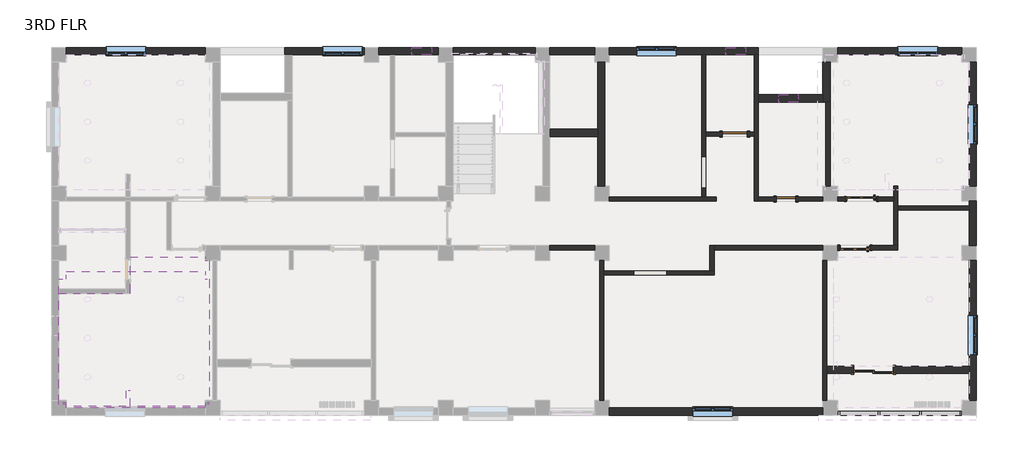
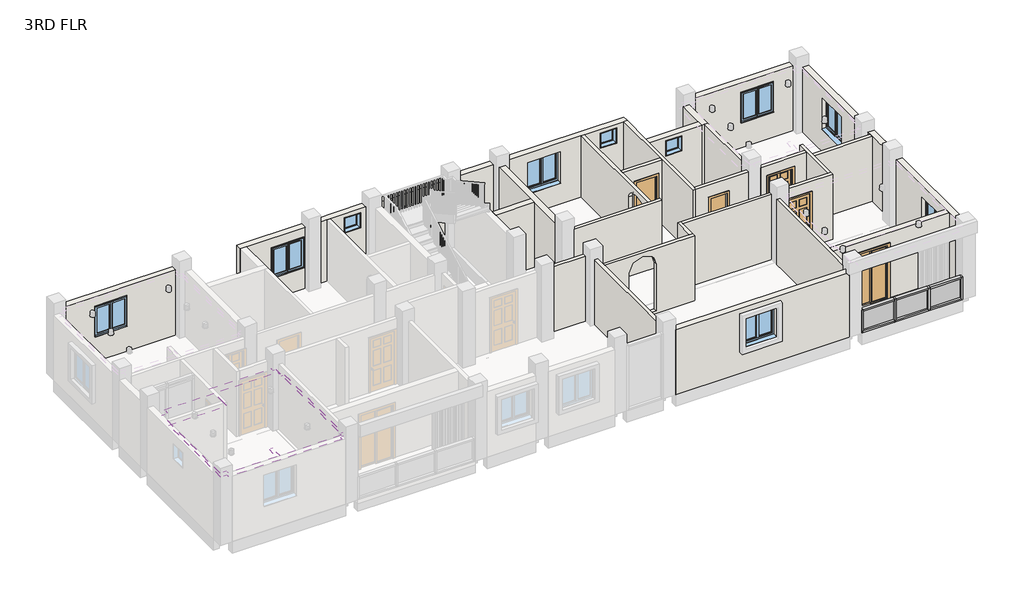
# One storey, part 2 of 5: 32 walls, 10 members, 10 windows, 5 doors, 3 plates, 2 coverings.
# Revit data of these elements (continued)
# Element 60 (IfcWindow, "w2.0001 : 4' X 4' WINDOW") (continued)
#   Materials on its faces: "Fenster - Kunststoff", "Fenster - Kunststoff weiss", "Glass", "Fenster - Holz"
# Element 61 (IfcWindow, "w2.0001 : 4' X 4' WINDOW")
#   Mark = "96"
#   Einbautiefe (von außen) = 0' - 5.51181"
#   Kippflügel = yes
#   Drehflügel im Grundriß darstellen = no
#   Drehflügel = yes
#   Rahmen = none
#   Glas = none
#   Flügel = none
#   Fensterbank innen = none
#   Fensterbank aussen = none
#   Phase Created = New Construction
#   Materials on its faces: "Fenster - Kunststoff", "Fenster - Kunststoff weiss", "Glass", "Fenster - Holz"
# Element 62 (IfcWindow, "w2.0001 : 4' X 4' WINDOW")
#   Mark = "103"
#   Einbautiefe (von außen) = 0' - 5.51181"
#   Kippflügel = yes
#   Drehflügel im Grundriß darstellen = no
#   Drehflügel = yes
#   Rahmen = none
#   Glas = none
#   Flügel = none
#   Fensterbank innen = none
#   Fensterbank aussen = none
#   Phase Created = New Construction
#   Materials on its faces: "Fenster - Kunststoff", "Fenster - Kunststoff weiss", "Glass", "Fenster - Holz"
# Materials
#   "WHITE CEILING 6\"": class "Generic", colour RGB 120 120 120, transparency 0, Cost = 0
#   "Glass": class "Glass", colour RGB 0 128 192, transparency 0.75, Description = "Soda Lime Glass", Cost = 0
#   "Wood - Birch - Solid Stained Light Low Gloss": class "Wood", colour RGB 210 159 95, transparency 0, Cost = 0
#   "Paint - Sienna": colour RGB 118 70 51, transparency 0, Cost = 0
#   "Cherry": class "Wood", colour RGB 226 177 128, transparency 0, Description = "Prunus Serotina", Cost = 0
#   "Aluminum": class "Metal", colour RGB 247 247 247, transparency 0, Description = "Aluminum 6061", Cost = 0
#   "Door - Panel": class "Wood", colour RGB 210 159 95, transparency 0, Cost = 0
#   "Door - Frame": colour RGB 118 70 51, transparency 0, Cost = 0
#   "SAND BEIGE PAINT": class "Generic", colour RGB 120 120 120, transparency 0, Cost = 0
#   "Sash": class "Wood", colour RGB 224 178 126, transparency 0, Cost = 0
#   "WINDOW FRAMING": class "Generic", colour RGB 120 120 120, transparency 0, Cost = 0
#   "Fenster - Kunststoff": colour RGB 249 249 249, transparency 0
#   "Fenster - Kunststoff weiss": colour RGB 249 249 249, transparency 0
#   "Fenster - Holz": colour RGB 216 135 75, transparency 0
